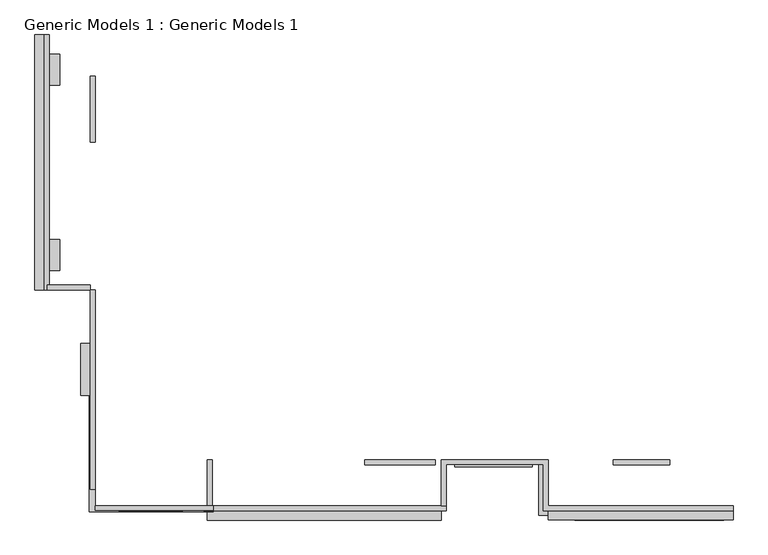
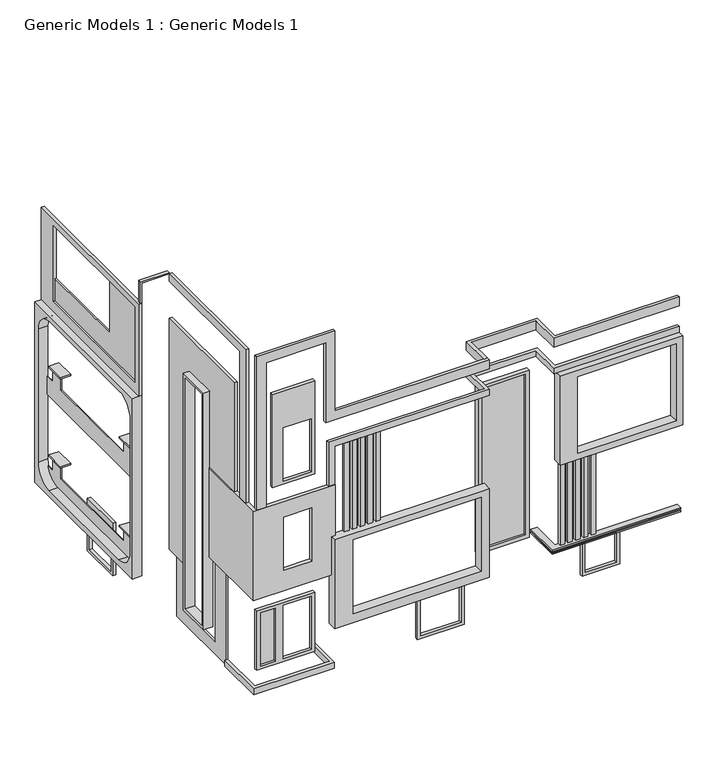
"""IFC4 building model written with IfcOpenShell, lengths in millimetres: proxy geometry, Generic Models 1 : Generic Models 1."""

from ifc_helpers import new_model, si_unit, point, frame, frame_2d, origin, place, context, project, spatial, polyline, circle_curve, trimmed, segment, composite_curve, outline, extrude, faceted_brep, source, transform, mapped, element, save


def generic_models_1_generic_models_1_784ad703(model_context):
    return source(origin(), model_context, "Body", "SolidModel", [
        extrude(outline(polyline([(2286.0, -3026.5394758), (2286.0, -4550.5394758), (762.0, -4550.5394758), (762.0, -3026.5394758), (2286.0, -3026.5394758)]), holes=[polyline([(2184.4, -3128.1394758), (863.6, -3128.1394758), (863.6, -4448.9394758), (2184.4, -4448.9394758), (2184.4, -3128.1394758)])]), frame((0.0, 3528.8495492, 0.0), z_axis=(0.0, 1.0, 0.0), x_axis=(0.0, 0.0, 1.0)), (0.0, 0.0, 1.0), 101.6),
        extrude(outline(polyline([(1066.8, 796.1605242), (1066.8, 2015.3605242), (2286.0, 2015.3605242), (2286.0, 796.1605242), (1066.8, 796.1605242)]), holes=[polyline([(2184.4, 1913.7605242), (1168.4, 1913.7605242), (1168.4, 897.7605242), (2184.4, 897.7605242), (2184.4, 1913.7605242)])]), frame((0.0, 3528.8495492, 0.0), z_axis=(0.0, 1.0, 0.0), x_axis=(0.0, 0.0, 1.0)), (0.0, 0.0, 1.0), 101.6),
        extrude(outline(polyline([(10463.0495492, 2616.2), (11885.4495492, 2616.2), (11885.4495492, 812.8), (10463.0495492, 812.8), (10463.0495492, 2616.2)]), holes=[polyline([(10564.6495492, 2133.6), (10564.6495492, 914.4), (11783.8495492, 914.4), (11783.8495492, 2133.6), (10564.6495492, 2133.6)])]), frame((-10443.3394758, 0.0, 0.0), z_axis=(1.0, 0.0, 0.0), x_axis=(0.0, 1.0, 0.0)), (0.0, 0.0, 1.0), 101.6),
        extrude(outline(polyline([(13106.4, -10443.3394758), (13150.85, -10443.3394758), (13150.85, -11376.7894758), (12420.6, -11376.7894758), (12420.6, -11332.3394758), (13106.4, -11332.3394758), (13106.4, -10443.3394758)])), frame((0.0, 7288.0495492, 0.0), z_axis=(0.0, 1.0, 0.0), x_axis=(0.0, 0.0, 1.0)), (0.0, 0.0, 1.0), 101.6),
        extrude(outline(polyline([(2992.7343966, 7837.7142857), (2992.7343966, 13106.4), (7288.0495492, 13106.4), (7288.0495492, 12861.2021482), (3306.4621615, 12861.2021482), (3306.4621615, 7837.7142857), (2992.7343966, 7837.7142857)])), frame((-10443.3394758, 0.0, 0.0), z_axis=(1.0, 0.0, 0.0), x_axis=(0.0, 1.0, 0.0)), (0.0, 0.0, 1.0), 101.6),
        extrude(outline(polyline([(-10443.3394758, 4163.8495492), (-10341.7394758, 4163.8495492), (-10341.7394758, 2639.8495492), (-7928.7394758, 2639.8495492), (-7928.7394758, 3630.4495492), (-7827.1394758, 3630.4495492), (-7827.1394758, 2538.2495492), (-10443.3394758, 2538.2495492), (-10443.3394758, 4163.8495492)])), frame((0.0, 0.0, 1538.5142857), z_axis=(0.0, 0.0, 1.0), x_axis=(1.0, 0.0, 0.0)), (0.0, 0.0, 1.0), 203.2),
        extrude(outline(polyline([(6475.2495492, 1981.2), (6475.2495492, 3657.6), (6964.1995492, 3657.6), (6964.1995492, 1538.5142857), (4163.8495492, 1538.5142857), (4163.8495492, 4789.7142857), (4773.4495492, 4789.7142857), (4773.4495492, 1981.2), (6475.2495492, 1981.2)])), frame((-10392.5394758, 0.0, 0.0), z_axis=(1.0, 0.0, 0.0), x_axis=(0.0, 1.0, 0.0)), (0.0, 0.0, 1.0), 50.8),
        extrude(outline(polyline([(12571.2495492, 6705.6), (12571.2495492, 6096.0), (7440.4495492, 6096.0), (7440.4495492, 6705.6), (7808.7495492, 6705.6), (7808.7495492, 7162.8), (8265.9495492, 7162.8), (8265.9495492, 6705.6), (11796.5495492, 6705.6), (11796.5495492, 7162.8), (12253.7495492, 7162.8), (12253.7495492, 6705.6), (12571.2495492, 6705.6)])), frame((-11357.7394758, 0.0, 0.0), z_axis=(1.0, 0.0, 0.0), x_axis=(0.0, 1.0, 0.0)), (0.0, 0.0, 1.0), 25.4),
        extrude(outline(polyline([(-11433.9394758, 12355.3495492), (-11103.7394758, 12355.3495492), (-11103.7394758, 11694.9495492), (-11433.9394758, 11694.9495492), (-11433.9394758, 12355.3495492)])), frame((0.0, 0.0, 7162.8), z_axis=(0.0, 0.0, 1.0), x_axis=(1.0, 0.0, 0.0)), (0.0, 0.0, 1.0), 50.8),
        extrude(outline(polyline([(-11433.9394758, 8367.5495492), (-11103.7394758, 8367.5495492), (-11103.7394758, 7707.1495492), (-11433.9394758, 7707.1495492), (-11433.9394758, 8367.5495492)])), frame((0.0, 0.0, 7162.8), z_axis=(0.0, 0.0, 1.0), x_axis=(1.0, 0.0, 0.0)), (0.0, 0.0, 1.0), 50.8),
        extrude(outline(polyline([(7516.6495492, 12192.0), (9015.2495492, 12192.0), (9015.2495492, 10363.2), (12088.6495492, 10363.2), (12088.6495492, 9601.2), (9015.2495492, 9601.2), (7516.6495492, 9601.2), (7516.6495492, 12192.0)])), frame((-11383.1394758, 0.0, 0.0), z_axis=(1.0, 0.0, 0.0), x_axis=(0.0, 1.0, 0.0)), (0.0, 0.0, 1.0), 50.8),
        extrude(outline(polyline([(-11433.9394758, 12355.3495492), (-11103.7394758, 12355.3495492), (-11103.7394758, 11694.9495492), (-11433.9394758, 11694.9495492), (-11433.9394758, 12355.3495492)])), frame((0.0, 0.0, 9144.0), z_axis=(0.0, 0.0, 1.0), x_axis=(1.0, 0.0, 0.0)), (0.0, 0.0, 1.0), 50.8),
        extrude(outline(polyline([(-11433.9394758, 8367.5495492), (-11103.7394758, 8367.5495492), (-11103.7394758, 7707.1495492), (-11433.9394758, 7707.1495492), (-11433.9394758, 8367.5495492)])), frame((0.0, 0.0, 9144.0), z_axis=(0.0, 0.0, 1.0), x_axis=(1.0, 0.0, 0.0)), (0.0, 0.0, 1.0), 50.8),
        extrude(outline(composite_curve([segment(trimmed(circle_curve(frame_2d((11961.6495492, 3860.8)), 609.6), [point((12536.385941, 3657.6))], [point((11961.6495492, 3251.2))], False, "CARTESIAN"), True, "CONTINUOUS"), segment(polyline([(11961.6495492, 3251.2), (8050.0495492, 3251.2)]), True, "CONTINUOUS"), segment(trimmed(circle_curve(frame_2d((8050.0495492, 3860.8)), 609.6), [point((8050.0495492, 3251.2))], [point((7475.3131575, 3657.6))], False, "CARTESIAN"), True, "CONTINUOUS"), segment(polyline([(7475.3131575, 3657.6), (7808.7495492, 3657.6), (7808.7495492, 4114.8), (8265.9495492, 4114.8), (8265.9495492, 3657.6), (11796.5495492, 3657.6), (11796.5495492, 4114.8), (12253.7495492, 4114.8), (12253.7495492, 3657.6), (12536.385941, 3657.6)]), True, "CONTINUOUS")], self_intersect=False)), frame((-11357.7394758, 0.0, 0.0), z_axis=(1.0, 0.0, 0.0), x_axis=(0.0, 1.0, 0.0)), (0.0, 0.0, 1.0), 25.4),
        extrude(outline(polyline([(-11433.9394758, 12355.3495492), (-11103.7394758, 12355.3495492), (-11103.7394758, 11694.9495492), (-11433.9394758, 11694.9495492), (-11433.9394758, 12355.3495492)])), frame((0.0, 0.0, 4114.8), z_axis=(0.0, 0.0, 1.0), x_axis=(1.0, 0.0, 0.0)), (0.0, 0.0, 1.0), 50.8),
        extrude(outline(polyline([(-11433.9394758, 8367.5495492), (-11103.7394758, 8367.5495492), (-11103.7394758, 7707.1495492), (-11433.9394758, 7707.1495492), (-11433.9394758, 8367.5495492)])), frame((0.0, 0.0, 4114.8), z_axis=(0.0, 0.0, 1.0), x_axis=(1.0, 0.0, 0.0)), (0.0, 0.0, 1.0), 50.8),
        faceted_brep([(-7801.7394758, 2538.2495492, 7837.7142857), (-8004.9394758, 2538.2495492, 7837.7142857), (-8004.9394758, 2639.8495492, 7837.7142857), (-7801.7394758, 2639.8495492, 7837.7142857), (-7801.7394758, 2538.2495492, 9144.0), (-2797.9394758, 2538.2495492, 9144.0), (-2797.9394758, 2538.2495492, 9347.2), (-8004.9394758, 2538.2495492, 9347.2), (-8004.9394758, 2639.8495492, 9347.2), (-2899.5394758, 2639.8495492, 9347.2), (-2899.5394758, 2639.8495492, 9144.0), (-7801.7394758, 2639.8495492, 9144.0), (-2797.9394758, 3528.8495492, 9347.2), (-702.4394758, 3528.8495492, 9347.2), (-702.4394758, 2538.2495492, 9347.2), (3374.2605242, 2538.2495492, 9347.2), (3374.2605242, 2639.8495492, 9347.2), (-600.8394758, 2639.8495492, 9347.2), (-600.8394758, 3630.4495492, 9347.2), (-2899.5394758, 3630.4495492, 9347.2), (-2899.5394758, 3630.4495492, 9144.0), (-600.8394758, 3630.4495492, 9144.0), (-600.8394758, 2639.8495492, 9144.0), (3374.2605242, 2639.8495492, 9144.0), (3374.2605242, 2538.2495492, 9144.0), (-702.4394758, 2538.2495492, 9144.0), (-702.4394758, 3528.8495492, 9144.0), (-2797.9394758, 3528.8495492, 9144.0)], [[[0, 1, 2, 3]], [[1, 0, 4, 5, 6, 7]], [[2, 1, 7, 8]], [[3, 2, 8, 9, 10, 11]], [[0, 3, 11, 4]], [[8, 7, 6, 12, 13, 14, 15, 16, 17, 18, 19, 9]], [[4, 11, 10, 20, 21, 22, 23, 24, 25, 26, 27, 5]], [[6, 5, 27, 12]], [[10, 9, 19, 20]], [[12, 27, 26, 13]], [[20, 19, 18, 21]], [[13, 26, 25, 14]], [[21, 18, 17, 22]], [[24, 23, 16, 15]], [[14, 25, 24, 15]], [[22, 17, 16, 23]]]),
        extrude(outline(polyline([(-489.7199817, 2534.4074171), (-489.7199817, 2639.8495492), (-346.8394758, 2639.8495492), (-346.8394758, 2534.4074171), (-489.7199817, 2534.4074171)])), frame((0.0, 0.0, 3181.35), z_axis=(0.0, 0.0, 1.0), x_axis=(1.0, 0.0, 0.0)), (0.0, 0.0, 1.0), 2914.65),
        extrude(outline(polyline([(-235.7199817, 2534.4074171), (-235.7199817, 2639.8495492), (-92.8394758, 2639.8495492), (-92.8394758, 2534.4074171), (-235.7199817, 2534.4074171)])), frame((0.0, 0.0, 3181.35), z_axis=(0.0, 0.0, 1.0), x_axis=(1.0, 0.0, 0.0)), (0.0, 0.0, 1.0), 2914.65),
        extrude(outline(polyline([(18.2800183, 2534.4074171), (18.2800183, 2639.8495492), (161.1605242, 2639.8495492), (161.1605242, 2534.4074171), (18.2800183, 2534.4074171)])), frame((0.0, 0.0, 3181.35), z_axis=(0.0, 0.0, 1.0), x_axis=(1.0, 0.0, 0.0)), (0.0, 0.0, 1.0), 2914.65),
        extrude(outline(polyline([(272.2800183, 2534.4074171), (272.2800183, 2639.8495492), (415.1605242, 2639.8495492), (415.1605242, 2534.4074171), (272.2800183, 2534.4074171)])), frame((0.0, 0.0, 3181.35), z_axis=(0.0, 0.0, 1.0), x_axis=(1.0, 0.0, 0.0)), (0.0, 0.0, 1.0), 2914.65),
        extrude(outline(polyline([(526.2800183, 2534.4074171), (526.2800183, 2639.8495492), (669.1605242, 2639.8495492), (669.1605242, 2534.4074171), (526.2800183, 2534.4074171)])), frame((0.0, 0.0, 3181.35), z_axis=(0.0, 0.0, 1.0), x_axis=(1.0, 0.0, 0.0)), (0.0, 0.0, 1.0), 2914.65),
        faceted_brep([(-804.0394758, 3630.4495492, 3181.35), (-600.8394758, 3630.4495492, 3181.35), (-600.8394758, 3630.4495492, 3048.0), (-804.0394758, 3630.4495492, 3048.0), (-804.0394758, 3630.4495492, 3089.275), (-784.9894758, 3630.4495492, 3089.275), (-784.9894758, 3630.4495492, 3140.075), (-804.0394758, 3630.4495492, 3140.075), (-804.0394758, 2436.6495492, 3181.35), (3374.2605242, 2436.6495492, 3181.35), (3374.2605242, 2639.8495492, 3181.35), (-600.8394758, 2639.8495492, 3181.35), (-600.8394758, 2639.8495492, 3048.0), (3374.2605242, 2639.8495492, 3048.0), (3374.2605242, 2436.6495492, 3048.0), (-804.0394758, 2436.6495492, 3048.0), (-804.0394758, 2436.6495492, 3089.275), (3374.2605242, 2436.6495492, 3089.275), (3374.2605242, 2455.6995492, 3089.275), (-784.9894758, 2455.6995492, 3089.275), (-784.9894758, 2455.6995492, 3140.075), (3374.2605242, 2455.6995492, 3140.075), (3374.2605242, 2436.6495492, 3140.075), (-804.0394758, 2436.6495492, 3140.075)], [[[0, 1, 2, 3, 4, 5, 6, 7]], [[1, 0, 8, 9, 10, 11]], [[2, 1, 11, 12]], [[3, 2, 12, 13, 14, 15]], [[4, 3, 15, 16]], [[5, 4, 16, 17, 18, 19]], [[6, 5, 19, 20]], [[7, 6, 20, 21, 22, 23]], [[0, 7, 23, 8]], [[9, 22, 21, 18, 17, 14, 13, 10]], [[12, 11, 10, 13]], [[16, 15, 14, 17]], [[20, 19, 18, 21]], [[8, 23, 22, 9]]]),
        extrude(outline(polyline([(-7342.1195524, 2639.8495492), (-7342.1195524, 2538.2495492), (-7494.5195524, 2538.2495492), (-7494.5195524, 2639.8495492), (-7342.1195524, 2639.8495492)])), frame((0.0, 0.0, 6096.0), z_axis=(0.0, 0.0, 1.0), x_axis=(1.0, 0.0, 0.0)), (0.0, 0.0, 1.0), 3048.0),
        extrude(outline(polyline([(-7088.1195524, 2639.8495492), (-7088.1195524, 2538.2495492), (-7240.5195524, 2538.2495492), (-7240.5195524, 2639.8495492), (-7088.1195524, 2639.8495492)])), frame((0.0, 0.0, 6096.0), z_axis=(0.0, 0.0, 1.0), x_axis=(1.0, 0.0, 0.0)), (0.0, 0.0, 1.0), 3048.0),
        extrude(outline(polyline([(-6834.1195524, 2639.8495492), (-6834.1195524, 2538.2495492), (-6986.5195524, 2538.2495492), (-6986.5195524, 2639.8495492), (-6834.1195524, 2639.8495492)])), frame((0.0, 0.0, 6096.0), z_axis=(0.0, 0.0, 1.0), x_axis=(1.0, 0.0, 0.0)), (0.0, 0.0, 1.0), 3048.0),
        extrude(outline(polyline([(-6580.1195524, 2639.8495492), (-6580.1195524, 2538.2495492), (-6732.5195524, 2538.2495492), (-6732.5195524, 2639.8495492), (-6580.1195524, 2639.8495492)])), frame((0.0, 0.0, 6096.0), z_axis=(0.0, 0.0, 1.0), x_axis=(1.0, 0.0, 0.0)), (0.0, 0.0, 1.0), 3048.0),
        extrude(outline(polyline([(-6326.1195524, 2639.8495492), (-6326.1195524, 2538.2495492), (-6478.5195524, 2538.2495492), (-6478.5195524, 2639.8495492), (-6326.1195524, 2639.8495492)])), frame((0.0, 0.0, 6096.0), z_axis=(0.0, 0.0, 1.0), x_axis=(1.0, 0.0, 0.0)), (0.0, 0.0, 1.0), 3048.0),
        extrude(outline(polyline([(-9735.5275058, 2614.4495492), (-10214.7394758, 2614.4495492), (-10214.7394758, 2639.8495492), (-9735.5275058, 2639.8495492), (-9735.5275058, 2614.4495492)])), frame((0.0, 0.0, 2438.4), z_axis=(0.0, 0.0, 1.0), x_axis=(1.0, 0.0, 0.0)), (0.0, 0.0, 1.0), 1828.8),
        extrude(outline(polyline([(2336.8, -10341.7394758), (2336.8, -8462.1394758), (4368.8, -8462.1394758), (4368.8, -10341.7394758), (2336.8, -10341.7394758)]), holes=[polyline([(4267.2, -8563.7394758), (2438.4, -8563.7394758), (2438.4, -9478.1394758), (4267.2, -9478.1394758), (4267.2, -8563.7394758)]), polyline([(4267.2, -9735.5275058), (2438.4, -9735.5275058), (2438.4, -10214.7394758), (4267.2, -10214.7394758), (4267.2, -9735.5275058)])]), frame((0.0, 2538.2495492, 0.0), z_axis=(0.0, 1.0, 0.0), x_axis=(0.0, 0.0, 1.0)), (0.0, 0.0, 1.0), 101.6),
        extrude(outline(polyline([(8432.8, -9833.7394758), (8432.8, -8462.1394758), (11633.2, -8462.1394758), (11633.2, -9833.7394758), (8432.8, -9833.7394758)]), holes=[polyline([(10363.2, -8563.7394758), (8534.4, -8563.7394758), (8534.4, -9478.1394758), (10363.2, -9478.1394758), (10363.2, -8563.7394758)])]), frame((0.0, 2538.2495492, 0.0), z_axis=(0.0, 1.0, 0.0), x_axis=(0.0, 0.0, 1.0)), (0.0, 0.0, 1.0), 101.6),
        extrude(outline(polyline([(12774.4495492, 12420.6), (12774.4495492, 9245.6), (7288.0495492, 9245.6), (7288.0495492, 12420.6), (12774.4495492, 12420.6)]), holes=[polyline([(12088.6495492, 12192.0), (7516.6495492, 12192.0), (7516.6495492, 9601.2), (12088.6495492, 9601.2), (12088.6495492, 12192.0)])]), frame((-11433.9394758, 0.0, 0.0), z_axis=(1.0, 0.0, 0.0), x_axis=(0.0, 1.0, 0.0)), (0.0, 0.0, 1.0), 101.6),
        faceted_brep([(-943.7394758, 3478.0495492, 8783.3566483), (-2607.4394758, 3478.0495492, 8783.3566483), (-2607.4394758, 3478.0495492, 3048.0), (-943.7394758, 3478.0495492, 3048.0), (-1070.7394758, 3478.0495492, 8687.7400791), (-1070.7394758, 3478.0495492, 3175.0), (-2480.4394758, 3478.0495492, 3175.0), (-2480.4394758, 3478.0495492, 8687.7400791), (-943.7394758, 3630.4495492, 8783.3566483), (-943.7394758, 3630.4495492, 3048.0), (-2607.4394758, 3630.4495492, 3048.0), (-2607.4394758, 3630.4495492, 8783.3566483), (-1070.7394758, 3554.2495492, 8687.7400791), (-2480.4394758, 3554.2495492, 8687.7400791), (-2480.4394758, 3554.2495492, 3175.0), (-1070.7394758, 3554.2495492, 3175.0)], [[[0, 1, 2, 3], [4, 5, 6, 7]], [[8, 9, 10, 11]], [[1, 0, 8, 11]], [[2, 1, 11, 10]], [[3, 2, 10, 9]], [[0, 3, 9, 8]], [[12, 13, 14, 15]], [[12, 15, 5, 4]], [[15, 14, 6, 5]], [[14, 13, 7, 6]], [[13, 12, 4, 7]]]),
        extrude(outline(polyline([(3374.2605242, 2639.8495492), (3374.2605242, 2538.2495492), (-702.4394758, 2538.2495492), (-702.4394758, 3528.8495492), (-2797.9394758, 3528.8495492), (-2797.9394758, 2639.8495492), (-2899.5394758, 2639.8495492), (-2899.5394758, 3630.4495492), (-600.8394758, 3630.4495492), (-600.8394758, 2639.8495492), (3374.2605242, 2639.8495492)])), frame((0.0, 0.0, 10058.4), z_axis=(0.0, 0.0, 1.0), x_axis=(1.0, 0.0, 0.0)), (0.0, 0.0, 1.0), 304.8),
        extrude(outline(polyline([(10363.2, -7801.7394758), (13106.4, -7801.7394758), (13106.4, -10341.7394758), (7837.7142857, -10341.7394758), (7837.7142857, -10036.9394758), (12801.6, -10036.9394758), (12801.6, -8106.5394758), (10058.4, -8106.5394758), (10058.4, -2797.9394758), (10363.2, -2797.9394758), (10363.2, -7801.7394758)])), frame((0.0, 2538.2495492, 0.0), z_axis=(0.0, 1.0, 0.0), x_axis=(0.0, 0.0, 1.0)), (0.0, 0.0, 1.0), 101.6),
        extrude(outline(polyline([(7288.0495492, 3657.6), (6132.3495492, 3657.6), (6132.3495492, 10464.8), (5014.7495492, 10464.8), (5014.7495492, 7837.7142857), (3630.4495492, 7837.7142857), (3630.4495492, 11582.4), (7288.0495492, 11582.4), (7288.0495492, 3657.6)])), frame((-10443.3394758, 0.0, 0.0), z_axis=(1.0, 0.0, 0.0), x_axis=(0.0, 1.0, 0.0)), (0.0, 0.0, 1.0), 101.6),
        faceted_brep([(-10468.7394758, 5014.7495492, 7837.7142857), (-10341.7394758, 5014.7495492, 7837.7142857), (-10341.7394758, 5014.7495492, 4789.7142857), (-10468.7394758, 5014.7495492, 4789.7142857), (-10468.7394758, 2512.8495492, 7837.7142857), (-7801.7394758, 2512.8495492, 7837.7142857), (-7801.7394758, 2639.8495492, 7837.7142857), (-10341.7394758, 2639.8495492, 7837.7142857), (-10341.7394758, 2639.8495492, 4789.7142857), (-7801.7394758, 2639.8495492, 4789.7142857), (-7801.7394758, 2512.8495492, 4789.7142857), (-10468.7394758, 2512.8495492, 4789.7142857), (-8563.7394758, 2639.8495492, 5486.4), (-8563.7394758, 2639.8495492, 7315.2), (-9478.1394758, 2639.8495492, 7315.2), (-9478.1394758, 2639.8495492, 5486.4), (-8563.7394758, 2512.8495492, 7315.2), (-8563.7394758, 2512.8495492, 5486.4), (-9478.1394758, 2512.8495492, 5486.4), (-9478.1394758, 2512.8495492, 7315.2)], [[[0, 1, 2, 3]], [[1, 0, 4, 5, 6, 7]], [[2, 1, 7, 8]], [[3, 2, 8, 9, 10, 11]], [[0, 3, 11, 4]], [[6, 5, 10, 9]], [[7, 6, 9, 8], [12, 13, 14, 15]], [[5, 4, 11, 10], [16, 17, 18, 19]], [[16, 13, 12, 17]], [[17, 12, 15, 18]], [[18, 15, 14, 19]], [[13, 16, 19, 14]]]),
        extrude(outline(polyline([(6132.3495492, 2336.8), (5014.7495492, 2336.8), (5014.7495492, 10464.8), (6132.3495492, 10464.8), (6132.3495492, 2336.8)]), holes=[polyline([(5116.3495492, 10363.2), (5116.3495492, 2438.4), (6030.7495492, 2438.4), (6030.7495492, 10363.2), (5116.3495492, 10363.2)])]), frame((-10646.5394758, 0.0, 0.0), z_axis=(1.0, 0.0, 0.0), x_axis=(0.0, 1.0, 0.0)), (0.0, 0.0, 1.0), 304.8),
        extrude(outline(polyline([(9144.0, -600.8394758), (6096.0, -600.8394758), (6096.0, 3374.2605242), (9144.0, 3374.2605242), (9144.0, -600.8394758)]), holes=[polyline([(8940.8, 3171.0605242), (6299.2, 3171.0605242), (6299.2, -29.3394758), (8940.8, -29.3394758), (8940.8, 3171.0605242)])]), frame((0.0, 2335.0495492, 0.0), z_axis=(0.0, 1.0, 0.0), x_axis=(0.0, 0.0, 1.0)), (0.0, 0.0, 1.0), 304.8),
        extrude(outline(polyline([(6096.0, -7928.7394758), (3048.0, -7928.7394758), (3048.0, -2899.5394758), (6096.0, -2899.5394758), (6096.0, -7928.7394758)]), holes=[polyline([(5892.8, -7323.6782102), (5892.8, -3166.2394758), (3352.8, -3166.2394758), (3352.8, -7323.6782102), (5892.8, -7323.6782102)])]), frame((0.0, 2335.0495492, 0.0), z_axis=(0.0, 1.0, 0.0), x_axis=(0.0, 0.0, 1.0)), (0.0, 0.0, 1.0), 304.8),
        extrude(outline(polyline([(12774.4495492, 9245.6), (12774.4495492, 3048.0), (7288.0495492, 3048.0), (7288.0495492, 9245.6), (12774.4495492, 9245.6)]), holes=[composite_curve([segment(trimmed(circle_curve(frame_2d((8050.0495492, 8432.8)), 609.6), [point((8050.0495492, 9042.4))], [point((7440.4495492, 8432.8))], True, "CARTESIAN"), True, "CONTINUOUS"), segment(polyline([(7440.4495492, 8432.8), (7440.4495492, 3860.8)]), True, "CONTINUOUS"), segment(trimmed(circle_curve(frame_2d((8050.0495492, 3860.8)), 609.6), [point((7440.4495492, 3860.8))], [point((8050.0495492, 3251.2))], True, "CARTESIAN"), True, "CONTINUOUS"), segment(polyline([(8050.0495492, 3251.2), (11961.6495492, 3251.2)]), True, "CONTINUOUS"), segment(trimmed(circle_curve(frame_2d((11961.6495492, 3860.8)), 609.6), [point((11961.6495492, 3251.2))], [point((12571.2495492, 3860.8))], True, "CARTESIAN"), True, "CONTINUOUS"), segment(polyline([(12571.2495492, 3860.8), (12571.2495492, 8432.8)]), True, "CONTINUOUS"), segment(trimmed(circle_curve(frame_2d((11961.6495492, 8432.8)), 609.6), [point((12571.2495492, 8432.8))], [point((11961.6495492, 9042.4))], True, "CARTESIAN"), True, "CONTINUOUS"), segment(polyline([(11961.6495492, 9042.4), (8050.0495492, 9042.4)]), True, "CONTINUOUS")], self_intersect=False)]), frame((-11637.1394758, 0.0, 0.0), z_axis=(1.0, 0.0, 0.0), x_axis=(0.0, 1.0, 0.0)), (0.0, 0.0, 1.0), 304.8),
    ])


if __name__ == "__main__":
    model = new_model("IFC4")
    model_context = context("Model", 3, world=origin())
    ifc_project = project(units=[si_unit("LENGTHUNIT", "METRE", prefix="MILLI")], contexts=[model_context])
    site = spatial("IfcSite", under=ifc_project)
    building = spatial("IfcBuilding", under=site)
    placement = place(None, origin())
    generic_models_1_generic_models_1_shape = generic_models_1_generic_models_1_784ad703(model_context)
    element("IfcBuildingElementProxy", 1, Name="Generic Models 1 : Generic Models 1", ObjectType="Generic Models 1 : Generic Models 1", at=placement, inside=building, context=model_context, shape_type="MappedRepresentation", body=[
        mapped(generic_models_1_generic_models_1_shape, transform((0.0, 0.0, 0.0), x_axis=(1.0, 0.0, 0.0), y_axis=(0.0, 1.0, 0.0), z_axis=(0.0, 0.0, 1.0))),
    ])
    save(model, "model.ifc")

# Revit data of these elements
# Element 1 (IfcBuildingElementProxy, "Generic Models 1 : Generic Models 1")
#   Materials on its faces: "02 white", "01 colour 1(1)", "01 brick", "01 wpc", "01 colour 1"
# Materials
#   "02 white": class "Generic", colour RGB 120 120 120, transparency 0, Cost = 0
#   "01 colour 1(1)": class "Generic", colour RGB 120 120 120, transparency 0, Cost = 0
#   "01 brick": class "Generic", colour RGB 120 120 120, transparency 0, Cost = 0
#   "01 wpc": class "Generic", colour RGB 120 120 120, transparency 0, Cost = 0
#   "01 colour 1": class "Generic", colour RGB 120 120 120, transparency 0, Cost = 0
